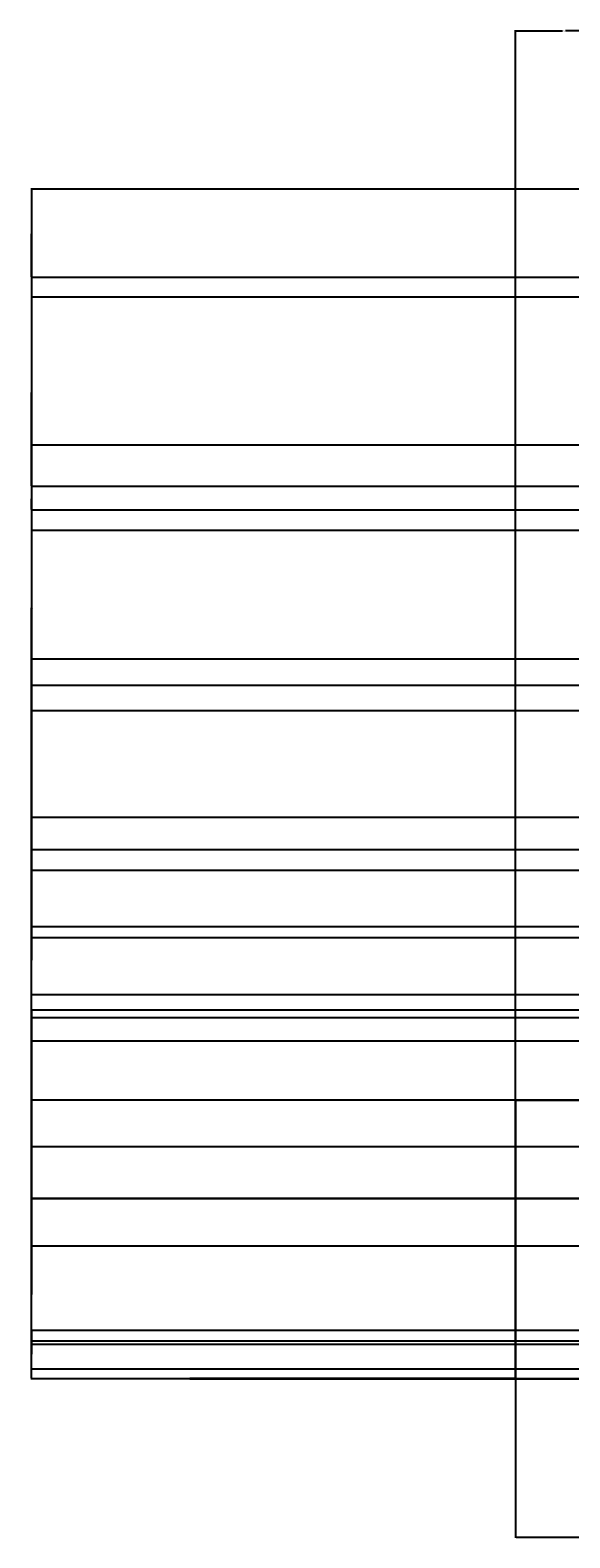
# Model space of a CAD drawing. Units: inches. Extents: x -14 to 886, y 45 to 435.
# Tile 1 of 5: x -14 to 125, y 45 to 435. Entities that reach past the tile are written whole.
import ezdxf

# ---------------------------------------------------------------- set-up
doc = ezdxf.new("R2010")
doc.units = ezdxf.units.IN
doc.header["$MEASUREMENT"] = 0
for name, color, linetype, lineweight in [('A-ANNO-DIMS', 2, 'Continuous', 18), ('C-TOPO', 7, 'Continuous', 35), ('L-WALL', 7, 'Continuous', 30)]:
    doc.layers.add(name, color=color, linetype=linetype, lineweight=lineweight)
doc.styles.get("Standard").update_dxf_attribs({"font": 'arial.ttf'})
doc.dimstyles.get("Standard").update_dxf_attribs({"dimtxt": 0.18, "dimasz": 0.18, "dimexe": 0.18, "dimexo": 0.0625, "dimgap": 0.09, "dimtad": 0, "dimtih": 1, "dimtoh": 1, "dimdec": 4, "dimzin": 0, "dimdsep": 46, "dimtxsty": 'Standard', "dimcen": 0.09, "dimadec": 0, "dimazin": 0, "dimtfac": 1, "dimtdec": 4, "dimtofl": 0, "dimtmove": 0, "dimatfit": 3, "dimfxl": 1, "dimtolj": 1, "dimtzin": 0, "dimarcsym": 0})

# ---------------------------------------------------------------- blocks, each defined once
blk = doc.blocks.new('*D16')
at = {"layer": 'A-ANNO-DIMS', "color": 0, "lineweight": -2, "transparency": 16777216}
for p, q in [((111.3, 86.48), (111.3, 45.47)), ((591.3, 86.48), (591.3, 45.47)), ((111.48, 45.65), (351.01, 45.65)), ((591.12, 45.65), (351.59, 45.65))]:
    blk.add_line(p, q, dxfattribs=at)
at = {"layer": 'A-ANNO-DIMS', "color": 0, "transparency": 16777216}
for points in [[(111.48, 45.68), (111.48, 45.62), (111.3, 45.65)], [(591.12, 45.68), (591.12, 45.62), (591.3, 45.65)]]:
    blk.add_solid(points, dxfattribs=at)
at = {"layer": 'Defpoints', "color": 0, "transparency": 16777216}
for p in [(111.3, 86.54), (591.3, 86.54), (591.3, 45.65)]:
    blk.add_point(p, dxfattribs=at)
at = {"layer": 'A-ANNO-DIMS', "color": 0, "transparency": 16777216, "insert": (351.3, 45.65), "char_height": 0.18, "attachment_point": 5}
blk.add_mtext('\\A1;480', dxfattribs=at)
blk = doc.blocks.new('*D17')
at = {"layer": 'A-ANNO-DIMS', "color": 0, "lineweight": -2, "transparency": 16777216}
for p, q in [((364.17, 393.98), (-13.96, 393.98)), ((-13.78, 393.8), (-13.78, 240.44)), ((-13.78, 86.72), (-13.78, 240.08)), ((111.24, 86.54), (-13.96, 86.54))]:
    blk.add_line(p, q, dxfattribs=at)
at = {"layer": 'A-ANNO-DIMS', "color": 0, "transparency": 16777216}
for points in [[(-13.81, 393.8), (-13.75, 393.8), (-13.78, 393.98)], [(-13.81, 86.72), (-13.75, 86.72), (-13.78, 86.54)]]:
    blk.add_solid(points, dxfattribs=at)
at = {"layer": 'Defpoints', "color": 0, "transparency": 16777216}
for p in [(-13.78, 393.98), (364.23, 393.98), (111.3, 86.54)]:
    blk.add_point(p, dxfattribs=at)
at = {"layer": 'A-ANNO-DIMS', "color": 0, "transparency": 16777216, "insert": (-13.78, 240.26), "char_height": 0.18, "attachment_point": 5}
blk.add_mtext('\\A1;307.44', dxfattribs=at)
blk = doc.blocks.new('*D18')
at = {"layer": 'A-ANNO-DIMS', "color": 0, "lineweight": -2, "transparency": 16777216}
for p, q in [((111.3, 86.48), (111.3, 45.47)), ((177.3, 86.48), (177.3, 45.47)), ((111.48, 45.65), (144.08, 45.65)), ((177.12, 45.65), (144.52, 45.65))]:
    blk.add_line(p, q, dxfattribs=at)
at = {"layer": 'A-ANNO-DIMS', "color": 0, "transparency": 16777216}
for points in [[(111.48, 45.68), (111.48, 45.62), (111.3, 45.65)], [(177.12, 45.68), (177.12, 45.62), (177.3, 45.65)]]:
    blk.add_solid(points, dxfattribs=at)
at = {"layer": 'Defpoints', "color": 0, "transparency": 16777216}
for p in [(111.3, 86.54), (177.3, 86.54), (177.3, 45.65)]:
    blk.add_point(p, dxfattribs=at)
at = {"layer": 'A-ANNO-DIMS', "color": 0, "transparency": 16777216, "insert": (144.3, 45.65), "char_height": 0.18, "attachment_point": 5}
blk.add_mtext('\\A1;66', dxfattribs=at)
blk = doc.blocks.new('*D24')
at = {"layer": 'A-ANNO-DIMS', "color": 0, "lineweight": -2, "transparency": 16777216}
for p, q in [((136.31, 311.03), (-13.96, 311.03)), ((-13.78, 310.85), (-13.78, 198.97)), ((-13.78, 86.72), (-13.78, 198.6)), ((195.24, 86.54), (-13.96, 86.54))]:
    blk.add_line(p, q, dxfattribs=at)
at = {"layer": 'A-ANNO-DIMS', "color": 0, "transparency": 16777216}
for points in [[(-13.81, 310.85), (-13.75, 310.85), (-13.78, 311.03)], [(-13.81, 86.72), (-13.75, 86.72), (-13.78, 86.54)]]:
    blk.add_solid(points, dxfattribs=at)
at = {"layer": 'Defpoints', "color": 0, "transparency": 16777216}
for p in [(-13.78, 311.03), (136.37, 311.03), (195.3, 86.54)]:
    blk.add_point(p, dxfattribs=at)
at = {"layer": 'A-ANNO-DIMS', "color": 0, "transparency": 16777216, "insert": (-13.78, 198.79), "char_height": 0.18, "attachment_point": 5}
blk.add_mtext('\\A1;224.5', dxfattribs=at)
blk = doc.blocks.new('*D26')
at = {"layer": 'A-ANNO-DIMS', "color": 0, "lineweight": -2, "transparency": 16777216}
for p, q in [((379.67, 366.03), (-13.96, 366.03)), ((-13.78, 365.85), (-13.78, 341.75)), ((-13.78, 317.28), (-13.78, 341.38)), ((136.31, 317.1), (-13.96, 317.1))]:
    blk.add_line(p, q, dxfattribs=at)
at = {"layer": 'A-ANNO-DIMS', "color": 0, "transparency": 16777216}
for points in [[(-13.81, 365.85), (-13.75, 365.85), (-13.78, 366.03)], [(-13.81, 317.28), (-13.75, 317.28), (-13.78, 317.1)]]:
    blk.add_solid(points, dxfattribs=at)
at = {"layer": 'Defpoints', "color": 0, "transparency": 16777216}
for p in [(-13.78, 366.03), (379.74, 366.03), (136.37, 317.1)]:
    blk.add_point(p, dxfattribs=at)
at = {"layer": 'A-ANNO-DIMS', "color": 0, "transparency": 16777216, "insert": (-13.78, 341.56), "char_height": 0.18, "attachment_point": 5}
blk.add_mtext('\\A1;48.92', dxfattribs=at)
blk = doc.blocks.new('*D27')
at = {"layer": 'A-ANNO-DIMS', "color": 0, "lineweight": -2, "transparency": 16777216}
for p, q in [((136.31, 317.1), (-13.96, 317.1)), ((-13.78, 316.92), (-13.78, 314.25)), ((-13.78, 311.21), (-13.78, 313.89)), ((136.31, 311.03), (-13.96, 311.03))]:
    blk.add_line(p, q, dxfattribs=at)
at = {"layer": 'A-ANNO-DIMS', "color": 0, "transparency": 16777216}
for points in [[(-13.81, 316.92), (-13.75, 316.92), (-13.78, 317.1)], [(-13.81, 311.21), (-13.75, 311.21), (-13.78, 311.03)]]:
    blk.add_solid(points, dxfattribs=at)
at = {"layer": 'Defpoints', "color": 0, "transparency": 16777216}
for p in [(-13.78, 317.1), (136.37, 317.1), (136.37, 311.03)]:
    blk.add_point(p, dxfattribs=at)
at = {"layer": 'A-ANNO-DIMS', "color": 0, "transparency": 16777216, "insert": (-13.78, 314.07), "char_height": 0.18, "attachment_point": 5}
blk.add_mtext('\\A1;6.069', dxfattribs=at)
blk = doc.blocks.new('*D29')
at = {"layer": 'A-ANNO-DIMS', "color": 0, "lineweight": -2, "transparency": 16777216}
for p, q in [((364.17, 393.98), (-13.96, 393.98)), ((-13.78, 393.8), (-13.78, 382.73)), ((-13.78, 371.29), (-13.78, 382.37)), ((549.29, 371.11), (-13.96, 371.11))]:
    blk.add_line(p, q, dxfattribs=at)
at = {"layer": 'A-ANNO-DIMS', "color": 0, "transparency": 16777216}
for points in [[(-13.81, 393.8), (-13.75, 393.8), (-13.78, 393.98)], [(-13.81, 371.29), (-13.75, 371.29), (-13.78, 371.11)]]:
    blk.add_solid(points, dxfattribs=at)
at = {"layer": 'Defpoints', "color": 0, "transparency": 16777216}
for p in [(364.23, 393.98), (-13.78, 371.11), (549.35, 371.11)]:
    blk.add_point(p, dxfattribs=at)
at = {"layer": 'A-ANNO-DIMS', "color": 0, "transparency": 16777216, "insert": (-13.78, 382.55), "char_height": 0.18, "attachment_point": 5}
blk.add_mtext('\\A1;22.865', dxfattribs=at)
blk = doc.blocks.new('*D32')
at = {"layer": 'A-ANNO-DIMS', "color": 0, "lineweight": -2, "transparency": 16777216}
for p, q in [((303.18, 327.78), (-13.96, 327.78)), ((-13.78, 327.6), (-13.78, 273.01)), ((-13.78, 218.06), (-13.78, 272.65)), ((303.18, 217.88), (-13.96, 217.88))]:
    blk.add_line(p, q, dxfattribs=at)
at = {"layer": 'A-ANNO-DIMS', "color": 0, "transparency": 16777216}
for points in [[(-13.81, 327.6), (-13.75, 327.6), (-13.78, 327.78)], [(-13.81, 218.06), (-13.75, 218.06), (-13.78, 217.88)]]:
    blk.add_solid(points, dxfattribs=at)
at = {"layer": 'Defpoints', "color": 0, "transparency": 16777216}
for p in [(-13.78, 327.78), (303.24, 327.78), (303.24, 217.88)]:
    blk.add_point(p, dxfattribs=at)
at = {"layer": 'A-ANNO-DIMS', "color": 0, "transparency": 16777216, "insert": (-13.78, 272.83), "char_height": 0.18, "attachment_point": 5}
blk.add_mtext('\\A1;109.9', dxfattribs=at)
blk = doc.blocks.new('*D35')
at = {"layer": 'A-ANNO-DIMS', "color": 0, "lineweight": -2, "transparency": 16777216}
for p, q in [((395.28, 217.88), (-13.96, 217.88)), ((-13.78, 217.7), (-13.78, 199.03)), ((-13.78, 180), (-13.78, 198.67)), ((395.28, 179.82), (-13.96, 179.82))]:
    blk.add_line(p, q, dxfattribs=at)
at = {"layer": 'A-ANNO-DIMS', "color": 0, "transparency": 16777216}
for points in [[(-13.81, 217.7), (-13.75, 217.7), (-13.78, 217.88)], [(-13.81, 180), (-13.75, 180), (-13.78, 179.82)]]:
    blk.add_solid(points, dxfattribs=at)
at = {"layer": 'Defpoints', "color": 0, "transparency": 16777216}
for p in [(-13.78, 217.88), (395.34, 217.88), (395.34, 179.82)]:
    blk.add_point(p, dxfattribs=at)
at = {"layer": 'A-ANNO-DIMS', "color": 0, "transparency": 16777216, "insert": (-13.78, 198.85), "char_height": 0.18, "attachment_point": 5}
blk.add_mtext('\\A1;38.06', dxfattribs=at)
blk = doc.blocks.new('*D36')
at = {"layer": 'A-ANNO-DIMS', "color": 0, "lineweight": -2, "transparency": 16777216}
for p, q in [((177.24, 179.82), (-13.96, 179.82)), ((-13.78, 179.64), (-13.78, 133.36)), ((-13.78, 86.72), (-13.78, 133)), ((177.24, 86.54), (-13.96, 86.54))]:
    blk.add_line(p, q, dxfattribs=at)
at = {"layer": 'A-ANNO-DIMS', "color": 0, "transparency": 16777216}
for points in [[(-13.81, 179.64), (-13.75, 179.64), (-13.78, 179.82)], [(-13.81, 86.72), (-13.75, 86.72), (-13.78, 86.54)]]:
    blk.add_solid(points, dxfattribs=at)
at = {"layer": 'Defpoints', "color": 0, "transparency": 16777216}
for p in [(-13.78, 179.82), (177.3, 179.82), (177.3, 86.54)]:
    blk.add_point(p, dxfattribs=at)
at = {"layer": 'A-ANNO-DIMS', "color": 0, "transparency": 16777216, "insert": (-13.78, 133.18), "char_height": 0.18, "attachment_point": 5}
blk.add_mtext('\\A1;93.28', dxfattribs=at)
blk = doc.blocks.new('*D37')
at = {"layer": 'A-ANNO-DIMS', "color": 0, "lineweight": -2, "transparency": 16777216}
for p, q in [((129.24, 146.54), (-13.96, 146.54)), ((-13.78, 146.36), (-13.78, 116.72)), ((-13.78, 86.72), (-13.78, 116.36)), ((129.24, 86.54), (-13.96, 86.54))]:
    blk.add_line(p, q, dxfattribs=at)
at = {"layer": 'A-ANNO-DIMS', "color": 0, "transparency": 16777216}
for points in [[(-13.81, 146.36), (-13.75, 146.36), (-13.78, 146.54)], [(-13.81, 86.72), (-13.75, 86.72), (-13.78, 86.54)]]:
    blk.add_solid(points, dxfattribs=at)
at = {"layer": 'Defpoints', "color": 0, "transparency": 16777216}
for p in [(-13.78, 146.54), (129.3, 146.54), (129.3, 86.54)]:
    blk.add_point(p, dxfattribs=at)
at = {"layer": 'A-ANNO-DIMS', "color": 0, "transparency": 16777216, "insert": (-13.78, 116.54), "char_height": 0.18, "attachment_point": 5}
blk.add_mtext('\\A1;60', dxfattribs=at)
blk = doc.blocks.new('*D38')
at = {"layer": 'A-ANNO-DIMS', "color": 0, "lineweight": -2, "transparency": 16777216}
for p, q in [((111.24, 158.54), (-13.96, 158.54)), ((-13.78, 158.36), (-13.78, 122.72)), ((-13.78, 86.72), (-13.78, 122.36)), ((111.24, 86.54), (-13.96, 86.54))]:
    blk.add_line(p, q, dxfattribs=at)
at = {"layer": 'A-ANNO-DIMS', "color": 0, "transparency": 16777216}
for points in [[(-13.81, 158.36), (-13.75, 158.36), (-13.78, 158.54)], [(-13.81, 86.72), (-13.75, 86.72), (-13.78, 86.54)]]:
    blk.add_solid(points, dxfattribs=at)
at = {"layer": 'Defpoints', "color": 0, "transparency": 16777216}
for p in [(-13.78, 158.54), (111.3, 158.54), (111.3, 86.54)]:
    blk.add_point(p, dxfattribs=at)
at = {"layer": 'A-ANNO-DIMS', "color": 0, "transparency": 16777216, "insert": (-13.78, 122.54), "char_height": 0.18, "attachment_point": 5}
blk.add_mtext('\\A1;72', dxfattribs=at)
blk = doc.blocks.new('*D41')
at = {"layer": 'A-ANNO-DIMS', "color": 0, "lineweight": -2, "transparency": 16777216}
for p, q in [((591.24, 259.14), (-13.96, 259.14)), ((-13.78, 258.96), (-13.78, 203.02)), ((-13.78, 146.72), (-13.78, 202.66)), ((537.19, 146.54), (-13.96, 146.54))]:
    blk.add_line(p, q, dxfattribs=at)
at = {"layer": 'A-ANNO-DIMS', "color": 0, "transparency": 16777216}
for points in [[(-13.81, 258.96), (-13.75, 258.96), (-13.78, 259.14)], [(-13.81, 146.72), (-13.75, 146.72), (-13.78, 146.54)]]:
    blk.add_solid(points, dxfattribs=at)
at = {"layer": 'Defpoints', "color": 0, "transparency": 16777216}
for p in [(-13.78, 259.14), (591.3, 259.14), (537.25, 146.54)]:
    blk.add_point(p, dxfattribs=at)
at = {"layer": 'A-ANNO-DIMS', "color": 0, "transparency": 16777216, "insert": (-13.78, 202.84), "char_height": 0.18, "attachment_point": 5}
blk.add_mtext('\\A1;112.6', dxfattribs=at)
blk = doc.blocks.new('*D42')
at = {"layer": 'A-ANNO-DIMS', "color": 0, "lineweight": -2, "transparency": 16777216}
for p, q in [((129.24, 272.54), (-13.96, 272.54)), ((-13.78, 272.36), (-13.78, 236.72)), ((-13.78, 200.72), (-13.78, 236.36)), ((129.24, 200.54), (-13.96, 200.54))]:
    blk.add_line(p, q, dxfattribs=at)
at = {"layer": 'A-ANNO-DIMS', "color": 0, "transparency": 16777216}
for points in [[(-13.81, 272.36), (-13.75, 272.36), (-13.78, 272.54)], [(-13.81, 200.72), (-13.75, 200.72), (-13.78, 200.54)]]:
    blk.add_solid(points, dxfattribs=at)
at = {"layer": 'Defpoints', "color": 0, "transparency": 16777216}
for p in [(-13.78, 272.54), (129.3, 272.54), (129.3, 200.54)]:
    blk.add_point(p, dxfattribs=at)
at = {"layer": 'A-ANNO-DIMS', "color": 0, "transparency": 16777216, "insert": (-13.78, 236.54), "char_height": 0.18, "attachment_point": 5}
blk.add_mtext('\\A1;72', dxfattribs=at)
blk = doc.blocks.new('*D44')
at = {"layer": 'A-ANNO-DIMS', "color": 0, "lineweight": -2, "transparency": 16777216}
for p, q in [((197.49, 133.16), (-13.96, 133.16)), ((-13.78, 132.98), (-13.78, 111.31)), ((-13.78, 89.26), (-13.78, 110.94)), ((197.49, 89.08), (-13.96, 89.08))]:
    blk.add_line(p, q, dxfattribs=at)
at = {"layer": 'A-ANNO-DIMS', "color": 0, "transparency": 16777216}
for points in [[(-13.81, 132.98), (-13.75, 132.98), (-13.78, 133.16)], [(-13.81, 89.26), (-13.75, 89.26), (-13.78, 89.08)]]:
    blk.add_solid(points, dxfattribs=at)
at = {"layer": 'Defpoints', "color": 0, "transparency": 16777216}
for p in [(-13.78, 133.16), (197.55, 133.16), (197.55, 89.08)]:
    blk.add_point(p, dxfattribs=at)
at = {"layer": 'A-ANNO-DIMS', "color": 0, "transparency": 16777216, "insert": (-13.78, 111.12), "char_height": 0.18, "attachment_point": 5}
blk.add_mtext('\\A1;44.08', dxfattribs=at)
blk = doc.blocks.new('*D49')
at = {"layer": 'A-ANNO-DIMS', "color": 0, "lineweight": -2, "transparency": 16777216}
for p, q in [((370.79, 203.37), (-13.96, 203.37)), ((-13.78, 203.19), (-13.78, 194.78)), ((-13.78, 186), (-13.78, 194.41)), ((370.79, 185.82), (-13.96, 185.82))]:
    blk.add_line(p, q, dxfattribs=at)
at = {"layer": 'A-ANNO-DIMS', "color": 0, "transparency": 16777216}
for points in [[(-13.81, 203.19), (-13.75, 203.19), (-13.78, 203.37)], [(-13.81, 186), (-13.75, 186), (-13.78, 185.82)]]:
    blk.add_solid(points, dxfattribs=at)
at = {"layer": 'Defpoints', "color": 0, "transparency": 16777216}
for p in [(-13.78, 203.37), (370.85, 203.37), (370.85, 185.82)]:
    blk.add_point(p, dxfattribs=at)
at = {"layer": 'A-ANNO-DIMS', "color": 0, "transparency": 16777216, "insert": (-13.78, 194.6), "char_height": 0.18, "attachment_point": 5}
blk.add_mtext('\\A1;17.55', dxfattribs=at)
blk = doc.blocks.new('*D53')
at = {"layer": 'A-ANNO-DIMS', "color": 0, "lineweight": -2, "transparency": 16777216}
for p, q in [((444.97, 305.77), (-13.96, 305.77)), ((-13.78, 305.59), (-13.78, 285.9)), ((-13.78, 265.85), (-13.78, 285.54)), ((444.97, 265.67), (-13.96, 265.67))]:
    blk.add_line(p, q, dxfattribs=at)
at = {"layer": 'A-ANNO-DIMS', "color": 0, "transparency": 16777216}
for points in [[(-13.81, 305.59), (-13.75, 305.59), (-13.78, 305.77)], [(-13.81, 265.85), (-13.75, 265.85), (-13.78, 265.67)]]:
    blk.add_solid(points, dxfattribs=at)
at = {"layer": 'Defpoints', "color": 0, "transparency": 16777216}
for p in [(-13.78, 305.77), (445.04, 305.77), (445.04, 265.67)]:
    blk.add_point(p, dxfattribs=at)
at = {"layer": 'A-ANNO-DIMS', "color": 0, "transparency": 16777216, "insert": (-13.78, 285.72), "char_height": 0.18, "attachment_point": 5}
blk.add_mtext('\\A1;40.104', dxfattribs=at)
blk = doc.blocks.new('*D54')
at = {"layer": 'A-ANNO-DIMS', "color": 0, "lineweight": -2, "transparency": 16777216}
for p, q in [((444.97, 181.83), (-13.96, 181.83)), ((-13.78, 181.65), (-13.78, 164.37)), ((-13.78, 146.72), (-13.78, 164)), ((444.97, 146.54), (-13.96, 146.54))]:
    blk.add_line(p, q, dxfattribs=at)
at = {"layer": 'A-ANNO-DIMS', "color": 0, "transparency": 16777216}
for points in [[(-13.81, 181.65), (-13.75, 181.65), (-13.78, 181.83)], [(-13.81, 146.72), (-13.75, 146.72), (-13.78, 146.54)]]:
    blk.add_solid(points, dxfattribs=at)
at = {"layer": 'Defpoints', "color": 0, "transparency": 16777216}
for p in [(-13.78, 181.83), (445.04, 181.83), (445.04, 146.54)]:
    blk.add_point(p, dxfattribs=at)
at = {"layer": 'A-ANNO-DIMS', "color": 0, "transparency": 16777216, "insert": (-13.78, 164.19), "char_height": 0.18, "attachment_point": 5}
blk.add_mtext('\\A1;35.29', dxfattribs=at)
blk = doc.blocks.new('*D55')
at = {"layer": 'A-ANNO-DIMS', "color": 0, "lineweight": -2, "transparency": 16777216}
for p, q in [((444.97, 265.67), (-13.96, 265.67)), ((-13.78, 265.49), (-13.78, 223.93)), ((-13.78, 182.01), (-13.78, 223.57)), ((444.97, 181.83), (-13.96, 181.83))]:
    blk.add_line(p, q, dxfattribs=at)
at = {"layer": 'A-ANNO-DIMS', "color": 0, "transparency": 16777216}
for points in [[(-13.81, 265.49), (-13.75, 265.49), (-13.78, 265.67)], [(-13.81, 182.01), (-13.75, 182.01), (-13.78, 181.83)]]:
    blk.add_solid(points, dxfattribs=at)
at = {"layer": 'Defpoints', "color": 0, "transparency": 16777216}
for p in [(-13.78, 265.67), (445.04, 265.67), (445.04, 181.83)]:
    blk.add_point(p, dxfattribs=at)
at = {"layer": 'A-ANNO-DIMS', "color": 0, "transparency": 16777216, "insert": (-13.78, 223.75), "char_height": 0.18, "attachment_point": 5}
blk.add_mtext('\\A1;83.84', dxfattribs=at)
blk = doc.blocks.new('*D57')
at = {"layer": 'A-ANNO-DIMS', "color": 0, "lineweight": -2, "transparency": 16777216}
for p, q in [((404, 99.06), (-13.96, 99.06)), ((-13.78, 98.88), (-13.78, 92.98)), ((-13.78, 86.72), (-13.78, 92.62)), ((391.73, 86.54), (-13.96, 86.54))]:
    blk.add_line(p, q, dxfattribs=at)
at = {"layer": 'A-ANNO-DIMS', "color": 0, "transparency": 16777216}
for points in [[(-13.81, 98.88), (-13.75, 98.88), (-13.78, 99.06)], [(-13.81, 86.72), (-13.75, 86.72), (-13.78, 86.54)]]:
    blk.add_solid(points, dxfattribs=at)
at = {"layer": 'Defpoints', "color": 0, "transparency": 16777216}
for p in [(404.07, 99.06), (-13.78, 86.54), (391.79, 86.54)]:
    blk.add_point(p, dxfattribs=at)
at = {"layer": 'A-ANNO-DIMS', "color": 0, "transparency": 16777216, "insert": (-13.78, 92.8), "char_height": 0.18, "attachment_point": 5}
blk.add_mtext('\\A1;12.52', dxfattribs=at)
blk = doc.blocks.new('*D60')
at = {"layer": 'A-ANNO-DIMS', "color": 0, "lineweight": -2, "transparency": 16777216}
for p, q in [((343.98, 231.64), (-13.96, 231.64)), ((-13.78, 231.46), (-13.78, 227.61)), ((-13.78, 223.39), (-13.78, 227.25)), ((343.98, 223.21), (-13.96, 223.21))]:
    blk.add_line(p, q, dxfattribs=at)
at = {"layer": 'A-ANNO-DIMS', "color": 0, "transparency": 16777216}
for points in [[(-13.81, 231.46), (-13.75, 231.46), (-13.78, 231.64)], [(-13.81, 223.39), (-13.75, 223.39), (-13.78, 223.21)]]:
    blk.add_solid(points, dxfattribs=at)
at = {"layer": 'Defpoints', "color": 0, "transparency": 16777216}
for p in [(-13.78, 231.64), (344.05, 231.64), (344.05, 223.21)]:
    blk.add_point(p, dxfattribs=at)
at = {"layer": 'A-ANNO-DIMS', "color": 0, "transparency": 16777216, "insert": (-13.78, 227.43), "char_height": 0.18, "attachment_point": 5}
blk.add_mtext('\\A1;8.424', dxfattribs=at)
blk = doc.blocks.new('*D62')
at = {"layer": 'A-ANNO-DIMS', "color": 0, "lineweight": -2, "transparency": 16777216}
for p, q in [((296.21, 173.82), (-13.96, 173.82)), ((-13.78, 173.64), (-13.78, 153.67)), ((-13.78, 133.34), (-13.78, 153.31)), ((296.21, 133.16), (-13.96, 133.16))]:
    blk.add_line(p, q, dxfattribs=at)
at = {"layer": 'A-ANNO-DIMS', "color": 0, "transparency": 16777216}
for points in [[(-13.81, 173.64), (-13.75, 173.64), (-13.78, 173.82)], [(-13.81, 133.34), (-13.75, 133.34), (-13.78, 133.16)]]:
    blk.add_solid(points, dxfattribs=at)
at = {"layer": 'Defpoints', "color": 0, "transparency": 16777216}
for p in [(-13.78, 173.82), (296.27, 173.82), (296.27, 133.16)]:
    blk.add_point(p, dxfattribs=at)
at = {"layer": 'A-ANNO-DIMS', "color": 0, "transparency": 16777216, "insert": (-13.78, 153.49), "char_height": 0.18, "attachment_point": 5}
blk.add_mtext('\\A1;40.66', dxfattribs=at)
blk = doc.blocks.new('*D64')
at = {"layer": 'A-ANNO-DIMS', "color": 0, "lineweight": -2, "transparency": 16777216}
for p, q in [((138.77, 133.07), (-13.96, 133.07)), ((-13.78, 132.89), (-13.78, 114.85)), ((-13.78, 96.45), (-13.78, 114.49)), ((138.77, 96.27), (-13.96, 96.27))]:
    blk.add_line(p, q, dxfattribs=at)
at = {"layer": 'A-ANNO-DIMS', "color": 0, "transparency": 16777216}
for points in [[(-13.81, 132.89), (-13.75, 132.89), (-13.78, 133.07)], [(-13.81, 96.45), (-13.75, 96.45), (-13.78, 96.27)]]:
    blk.add_solid(points, dxfattribs=at)
at = {"layer": 'Defpoints', "color": 0, "transparency": 16777216}
for p in [(-13.78, 133.07), (138.83, 133.07), (138.83, 96.27)]:
    blk.add_point(p, dxfattribs=at)
at = {"layer": 'A-ANNO-DIMS', "color": 0, "transparency": 16777216, "insert": (-13.78, 114.67), "char_height": 0.18, "attachment_point": 5}
blk.add_mtext('\\A1;36.8', dxfattribs=at)
blk = doc.blocks.new('*D65')
at = {"layer": 'A-ANNO-DIMS', "color": 0, "lineweight": -2, "transparency": 16777216}
for p, q in [((111.3, 158.6), (111.3, 435.05)), ((111.48, 434.87), (123.44, 434.87)), ((136.19, 434.87), (124.23, 434.87)), ((136.37, 158.6), (136.37, 435.05))]:
    blk.add_line(p, q, dxfattribs=at)
at = {"layer": 'A-ANNO-DIMS', "color": 0, "transparency": 16777216}
for points in [[(111.48, 434.9), (111.48, 434.84), (111.3, 434.87)], [(136.19, 434.9), (136.19, 434.84), (136.37, 434.87)]]:
    blk.add_solid(points, dxfattribs=at)
at = {"layer": 'Defpoints', "color": 0, "transparency": 16777216}
for p in [(136.37, 434.87), (111.3, 158.54), (136.37, 158.54)]:
    blk.add_point(p, dxfattribs=at)
at = {"layer": 'A-ANNO-DIMS', "color": 0, "transparency": 16777216, "insert": (123.84, 434.87), "char_height": 0.18, "attachment_point": 5}
blk.add_mtext('\\A1;25.07', dxfattribs=at)
blk = doc.blocks.new('*D68')
at = {"layer": 'A-ANNO-DIMS', "color": 0, "lineweight": -2, "transparency": 16777216}
for p, q in [((196.33, 120.82), (-13.96, 120.82)), ((-13.78, 120.64), (-13.78, 108.32)), ((-13.78, 95.64), (-13.78, 107.96)), ((196.33, 95.46), (-13.96, 95.46))]:
    blk.add_line(p, q, dxfattribs=at)
at = {"layer": 'A-ANNO-DIMS', "color": 0, "transparency": 16777216}
for points in [[(-13.81, 120.64), (-13.75, 120.64), (-13.78, 120.82)], [(-13.81, 95.64), (-13.75, 95.64), (-13.78, 95.46)]]:
    blk.add_solid(points, dxfattribs=at)
at = {"layer": 'Defpoints', "color": 0, "transparency": 16777216}
for p in [(-13.78, 120.82), (196.39, 120.82), (196.39, 95.46)]:
    blk.add_point(p, dxfattribs=at)
at = {"layer": 'A-ANNO-DIMS', "color": 0, "transparency": 16777216, "insert": (-13.78, 108.14), "char_height": 0.18, "attachment_point": 5}
blk.add_mtext('\\A1;25.356', dxfattribs=at)

msp = doc.modelspace()

# ---------------------------------------------------------------- linework, layer by layer
at = {"layer": 'C-TOPO'}
msp.add_line((111.3024, 86.5389), (27.1131, 86.5389), dxfattribs=at)
at = {"layer": 'L-WALL'}
msp.add_lwpolyline([(129.3024, 86.5389), (129.3024, 158.5389), (111.3024, 158.5389), (111.3024, 86.5389), (379.7908, 86.5389), (379.7908, 179.8201)], dxfattribs=at)

# ---------------------------------------------------------------- dimensions: what is measured, and where the dimension line sits
at = {"layer": 'A-ANNO-DIMS'}
for base, p1, p2, override, picture, middle in [((136.3714, 434.8697), (111.3024, 158.5389), (136.3714, 158.5389), {"dimdec": 2, "dimlfac": 1, "dimrnd": 0, "dimzin": 0, "dimdsep": 46, "dimlunit": 2}, '*D65', (123.8369, 434.8697)), ((591.3024, 45.6489), (111.3024, 86.5389), (591.3024, 86.5389), {"dimdec": 0, "dimlfac": 1, "dimrnd": 0, "dimzin": 0, "dimdsep": 46, "dimlunit": 2}, '*D16', (351.3024, 45.6489)), ((177.3024, 45.6489), (111.3024, 86.5389), (177.3024, 86.5389), {"dimdec": 0, "dimlfac": 1, "dimrnd": 0, "dimzin": 0, "dimdsep": 46, "dimlunit": 2}, '*D18', (144.3024, 45.6489))]:
    dim = msp.add_linear_dim(base=base, p1=p1, p2=p2, dimstyle='Standard', override=override, dxfattribs=at)
    dim.commit()
    dim.dimension.update_dxf_attribs({"geometry": picture, "text_midpoint": middle})
for base, p1, p2, override, picture, middle in [((-13.7769, 393.9797), (111.3024, 86.5389), (364.2304, 393.9797), {"dimdec": 2, "dimlfac": 1, "dimrnd": 0, "dimzin": 0, "dimdsep": 46, "dimlunit": 2}, '*D17', (-13.7769, 240.2593)), ((-13.7769, 371.1143), (364.2304, 393.9797), (549.3534, 371.1143), {"dimdec": 3, "dimlfac": 1, "dimrnd": 0, "dimzin": 0, "dimdsep": 46, "dimlunit": 2}, '*D29', (-13.7769, 382.547)), ((-13.7769, 366.0265), (136.3714, 317.1024), (379.7355, 366.0265), {"dimdec": 2, "dimlfac": 1, "dimrnd": 0, "dimzin": 0, "dimdsep": 46, "dimlunit": 2}, '*D26', (-13.7769, 341.5645)), ((-13.7769, 327.7815), (303.2386, 217.8839), (303.2386, 327.7815), {"dimdec": 1, "dimlfac": 1, "dimrnd": 0, "dimzin": 0, "dimdsep": 46, "dimlunit": 2}, '*D32', (-13.7769, 272.8327)), ((-13.7769, 317.1024), (136.3714, 311.0336), (136.3714, 317.1024), {"dimdec": 3, "dimlfac": 1, "dimrnd": 0, "dimzin": 0, "dimdsep": 46, "dimlunit": 2}, '*D27', (-13.7769, 314.068)), ((-13.7769, 311.0336), (195.3024, 86.5389), (136.3714, 311.0336), {"dimdec": 1, "dimlfac": 1, "dimrnd": 0, "dimzin": 0, "dimdsep": 46, "dimlunit": 2}, '*D24', (-13.7769, 198.7862)), ((-13.7769, 305.7727), (445.0372, 265.6686), (445.0372, 305.7727), {"dimdec": 3, "dimlfac": 1, "dimrnd": 0, "dimzin": 0, "dimdsep": 46, "dimlunit": 2}, '*D53', (-13.7769, 285.7207)), ((-13.7769, 272.5389), (129.3024, 200.5389), (129.3024, 272.5389), {"dimdec": 0, "dimlfac": 1, "dimrnd": 0, "dimzin": 0, "dimdsep": 46, "dimlunit": 2}, '*D42', (-13.7769, 236.5389)), ((-13.7769, 265.6686), (445.0372, 181.8319), (445.0372, 265.6686), {"dimdec": 2, "dimlfac": 1, "dimrnd": 0, "dimzin": 0, "dimdsep": 46, "dimlunit": 2}, '*D55', (-13.7769, 223.7503)), ((-13.7769, 259.1435), (537.2506, 146.5389), (591.3024, 259.1435), {"dimdec": 1, "dimlfac": 1, "dimrnd": 0, "dimzin": 0, "dimdsep": 46, "dimlunit": 2}, '*D41', (-13.7769, 202.8412)), ((-13.7769, 231.6392), (344.045, 223.215), (344.045, 231.6392), {"dimdec": 3, "dimlfac": 1, "dimrnd": 0, "dimzin": 0, "dimdsep": 46, "dimlunit": 2}, '*D60', (-13.7769, 227.4271)), ((-13.7769, 217.8839), (395.3394, 179.8201), (395.3394, 217.8839), {"dimdec": 2, "dimlfac": 1, "dimrnd": 0, "dimzin": 0, "dimdsep": 46, "dimlunit": 2}, '*D35', (-13.7769, 198.852)), ((-13.7769, 203.3712), (370.8507, 185.8201), (370.8507, 203.3712), {"dimdec": 2, "dimlfac": 1, "dimrnd": 0, "dimzin": 0, "dimdsep": 46, "dimlunit": 2}, '*D49', (-13.7769, 194.5957)), ((-13.7769, 181.8319), (445.0372, 146.5389), (445.0372, 181.8319), {"dimdec": 2, "dimlfac": 1, "dimrnd": 0, "dimzin": 0, "dimdsep": 46, "dimlunit": 2}, '*D54', (-13.7769, 164.1854)), ((-13.7769, 179.8201), (177.3024, 86.5389), (177.3024, 179.8201), {"dimdec": 2, "dimlfac": 1, "dimrnd": 0, "dimzin": 0, "dimdsep": 46, "dimlunit": 2}, '*D36', (-13.7769, 133.1795)), ((-13.7769, 173.8201), (296.2693, 133.1624), (296.2693, 173.8201), {"dimdec": 2, "dimlfac": 1, "dimrnd": 0, "dimzin": 0, "dimdsep": 46, "dimlunit": 2}, '*D62', (-13.7769, 153.4913)), ((-13.7769, 158.5389), (111.3024, 86.5389), (111.3024, 158.5389), {"dimdec": 0, "dimlfac": 1, "dimrnd": 0, "dimzin": 0, "dimdsep": 46, "dimlunit": 2}, '*D38', (-13.7769, 122.5389)), ((-13.7769, 146.5389), (129.3024, 86.5389), (129.3024, 146.5389), {"dimdec": 0, "dimlfac": 1, "dimrnd": 0, "dimzin": 0, "dimdsep": 46, "dimlunit": 2}, '*D37', (-13.7769, 116.5389)), ((-13.7769, 133.1624), (197.5542, 89.0847), (197.5542, 133.1624), {"dimdec": 2, "dimlfac": 1, "dimrnd": 0, "dimzin": 0, "dimdsep": 46, "dimlunit": 2}, '*D44', (-13.7769, 111.1236)), ((-13.7769, 133.0686), (138.8348, 96.2678), (138.8348, 133.0686), {"dimdec": 1, "dimlfac": 1, "dimrnd": 0, "dimzin": 0, "dimdsep": 46, "dimlunit": 2}, '*D64', (-13.7769, 114.6682)), ((-13.7769, 120.8171), (196.3935, 95.4612), (196.3935, 120.8171), {"dimdec": 3, "dimlfac": 1, "dimrnd": 0, "dimzin": 0, "dimdsep": 46, "dimlunit": 2}, '*D68', (-13.7769, 108.1391)), ((-13.7769, 86.5389), (404.0655, 99.0583), (391.7908, 86.5389), {"dimdec": 2, "dimlfac": 1, "dimrnd": 0, "dimzin": 0, "dimdsep": 46, "dimlunit": 2}, '*D57', (-13.7769, 92.7986))]:
    dim = msp.add_linear_dim(base=base, p1=p1, p2=p2, angle=90, dimstyle='Standard', override=override, dxfattribs=at)
    dim.commit()
    dim.dimension.update_dxf_attribs({"geometry": picture, "text_midpoint": middle})

doc.saveas('drawing.dxf')
